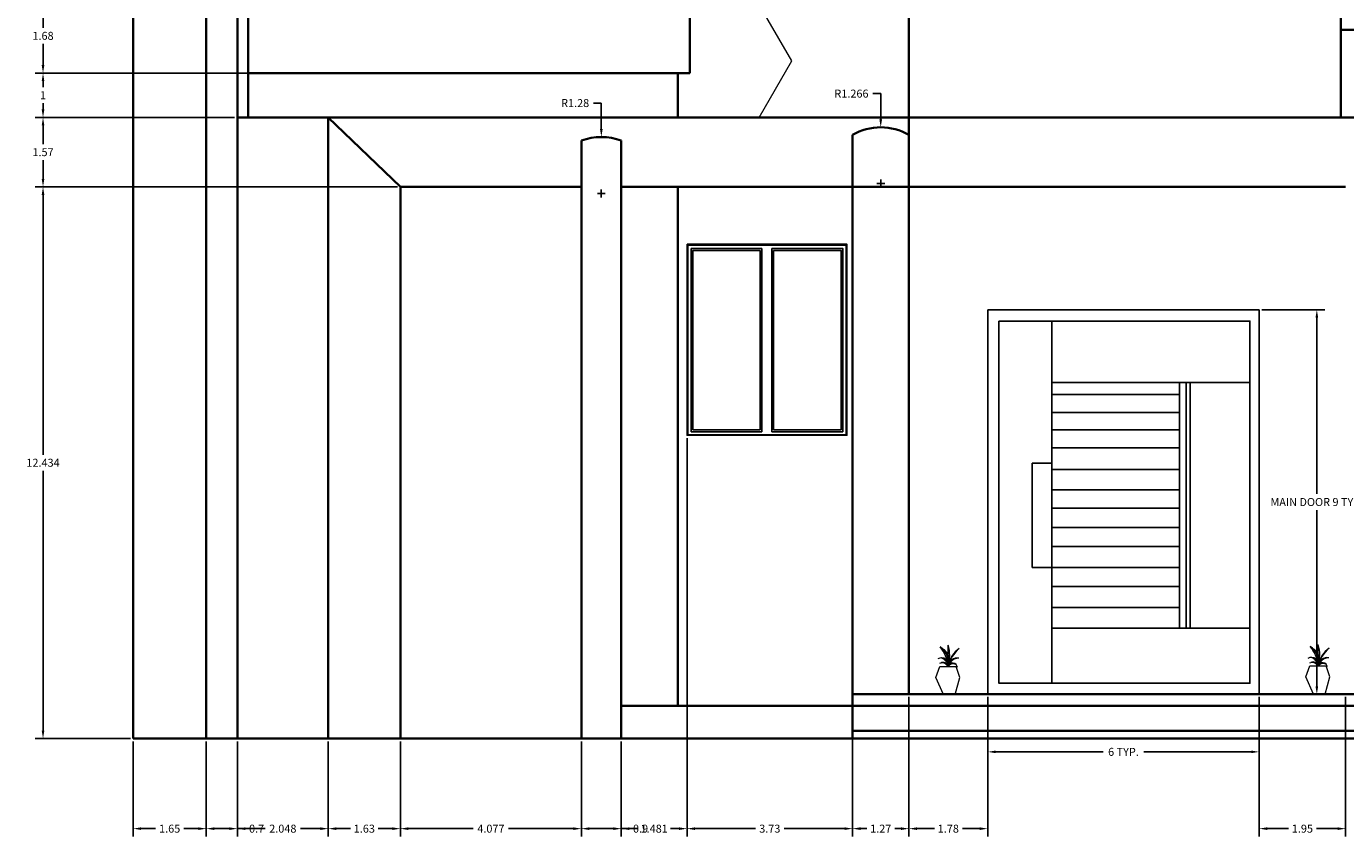
# Model space of a CAD drawing. Units: millimetres. Extents: x 2521.2 to 2565.9, y 755.2 to 798.1.
# Tile 1 of 3: x 2521.2 to 2550.9, y 755.2 to 773.4. Entities that reach past the tile are written whole.
import ezdxf

# ---------------------------------------------------------------- set-up
doc = ezdxf.new("R2010")
doc.units = ezdxf.units.MM
for name, color, linetype, lineweight in [('A-ANNO-DIMS', 2, 'Continuous', 18), ('A-DOOR', 3, 'Continuous', 25), ('A-ELEV', 7, 'Continuous', 35), ('A-GLAZ', 4, 'Continuous', 25), ('A-WALL-PATT', 8, 'Continuous', 13), ('L-PLNT', 3, 'Continuous', 18)]:
    doc.layers.add(name, color=color, linetype=linetype, lineweight=lineweight)
doc.styles.get("Standard").update_dxf_attribs({"font": 'arial.ttf'})
doc.dimstyles.get("Standard").update_dxf_attribs({"dimtxt": 0.18, "dimasz": 0.18, "dimexe": 0.18, "dimexo": 0.0625, "dimgap": 0.09, "dimtad": 0, "dimtih": 1, "dimtoh": 1, "dimdec": 4, "dimzin": 0, "dimdsep": 46, "dimtxsty": 'Standard', "dimcen": 0.09, "dimadec": 0, "dimazin": 0, "dimtfac": 1, "dimtdec": 4, "dimtofl": 0, "dimtmove": 0, "dimatfit": 3, "dimfxl": 1, "dimtolj": 1, "dimtzin": 0, "dimarcsym": 0})

# ---------------------------------------------------------------- blocks, each defined once
blk = doc.blocks.new('WIN-DOUBLE')
for p, q in [((2559.456, 776.3), (2559.456, 780.343)), ((2559.491, 780.386), (2559.491, 776.258)), ((2559.716, 776.3), (2559.716, 780.386)), ((2559.756, 776.3), (2559.756, 780.343)), ((2559.716, 776.3), (2559.716, 776.258)), ((2559.716, 776.258), (2561.319, 776.258))]:
    blk.add_line(p, q)
for points in [[(2557.805, 780.483), (2561.406, 780.483), (2561.406, 776.176), (2557.805, 776.176)], [(2557.825, 780.462), (2561.393, 780.462), (2561.393, 776.189), (2557.825, 776.189)]]:
    blk.add_lwpolyline(points, close=True)
for points in [[(2559.491, 776.258), (2557.898, 776.258), (2557.898, 780.386), (2559.491, 780.386)], [(2559.456, 776.3), (2557.936, 776.3), (2557.936, 780.343), (2559.456, 780.343)], [(2559.716, 780.386), (2561.319, 780.386), (2561.319, 776.258)], [(2559.756, 780.343), (2561.276, 780.343), (2561.276, 776.3), (2559.756, 776.3)]]:
    blk.add_lwpolyline(points)
blk = doc.blocks.new('DOOR-MAIN')
for p, q in [((2542.828, 758.373), (2542.828, 767.037)), ((2542.828, 767.037), (2548.944, 767.037)), ((2548.944, 767.037), (2548.944, 758.373)), ((2544.274, 766.783), (2544.274, 758.62)), ((2544.274, 765.396), (2548.734, 765.396)), ((2547.145, 765.132), (2544.274, 765.132)), ((2547.145, 765.396), (2547.145, 759.865)), ((2547.299, 765.396), (2547.299, 759.865)), ((2547.389, 765.396), (2547.389, 759.865)), ((2547.145, 764.725), (2544.274, 764.725)), ((2547.145, 764.331), (2544.274, 764.331)), ((2547.145, 763.924), (2544.274, 763.924)), ((2543.829, 761.227), (2543.829, 763.581)), ((2543.829, 763.581), (2544.274, 763.581)), ((2547.145, 763.441), (2544.274, 763.441)), ((2547.145, 762.983), (2544.274, 762.983)), ((2547.145, 762.564), (2544.274, 762.564)), ((2547.145, 762.131), (2544.274, 762.131)), ((2547.145, 761.699), (2544.274, 761.699)), ((2544.274, 761.227), (2543.829, 761.227)), ((2547.145, 761.227), (2544.274, 761.227)), ((2547.145, 760.804), (2544.274, 760.804)), ((2547.145, 760.33), (2544.274, 760.33)), ((2544.274, 759.865), (2548.734, 759.865))]:
    blk.add_line(p, q)
blk.add_lwpolyline([(2543.079, 766.783), (2548.734, 766.783), (2548.734, 758.62), (2543.079, 758.62)], close=True)
blk = doc.blocks.new('PLANTER')
for p, q in [((2558.646, 757.758), (2558.737, 758.005)), ((2558.737, 758.005), (2559.107, 758.005)), ((2559.189, 757.758), (2559.107, 758.005)), ((2558.817, 757.373), (2558.646, 757.758)), ((2559.08, 757.373), (2559.189, 757.758))]:
    blk.add_line(p, q)
for centre, radius, start, end in [((2558.504, 758.092), 0.427, 348.2161, 55.5831), ((2558.151, 757.944), 0.777, 5.6498, 40.0889), ((2558.161, 757.954), 0.763, 3.8104, 39.9888), ((2558.66, 758.146), 0.293, 333.1798, 63.2065), ((2558.164, 758.26), 0.796, 342.0282, 16.5628), ((2559.557, 757.89), 0.648, 126.493, 168.9551), ((2530.529, 758.527), 28.398, 358.9459, 359.9172), ((2559.736, 757.784), 0.843, 132.0051, 164.8224), ((2558.772, 758.043), 0.155, 345.7039, 120.8927), ((2558.788, 757.931), 0.154, 28.8769, 113.7957), ((2558.813, 757.985), 0.111, 10.1799, 119.9068), ((2558.697, 757.984), 0.226, 5.301, 71.0335), ((2559.127, 757.986), 0.208, 79.6534, 172.2119), ((2559.023, 757.968), 0.112, 7.4318, 155.8017), ((2559.176, 757.925), 0.266, 92.441, 162.4192), ((2559.033, 757.927), 0.136, 55.8779, 144.8755)]:
    blk.add_arc(centre, radius, start, end)
blk = doc.blocks.new('*D6')
at = {"layer": 'A-ANNO-DIMS', "color": 0, "lineweight": -2, "transparency": 16777216}
for p, q in [((2549.006, 767.037), (2550.423, 767.037)), ((2550.243, 766.857), (2550.243, 762.888)), ((2550.243, 758.553), (2550.243, 762.522)), ((2549.006, 758.373), (2550.423, 758.373))]:
    blk.add_line(p, q, dxfattribs=at)
at = {"layer": 'A-ANNO-DIMS', "color": 0, "transparency": 16777216}
for points in [[(2550.213, 766.857), (2550.273, 766.857), (2550.243, 767.037)], [(2550.213, 758.553), (2550.273, 758.553), (2550.243, 758.373)]]:
    blk.add_solid(points, dxfattribs=at)
at = {"layer": 'Defpoints', "color": 0, "transparency": 16777216}
for p in [(2548.944, 767.037), (2550.243, 767.037), (2548.944, 758.373)]:
    blk.add_point(p, dxfattribs=at)
at = {"layer": 'A-ANNO-DIMS', "color": 0, "transparency": 16777216, "insert": (2550.243, 762.705), "char_height": 0.18, "attachment_point": 5}
blk.add_mtext('\\A1;MAIN DOOR 9 TYP.', dxfattribs=at)
blk = doc.blocks.new('*D7')
at = {"layer": 'A-ANNO-DIMS', "color": 0, "lineweight": -2, "transparency": 16777216}
for p, q in [((2542.828, 758.311), (2542.828, 756.894)), ((2548.944, 758.311), (2548.944, 756.894)), ((2543.008, 757.074), (2545.427, 757.074)), ((2548.764, 757.074), (2546.344, 757.074))]:
    blk.add_line(p, q, dxfattribs=at)
at = {"layer": 'A-ANNO-DIMS', "color": 0, "transparency": 16777216}
for points in [[(2543.008, 757.104), (2543.008, 757.044), (2542.828, 757.074)], [(2548.764, 757.104), (2548.764, 757.044), (2548.944, 757.074)]]:
    blk.add_solid(points, dxfattribs=at)
at = {"layer": 'Defpoints', "color": 0, "transparency": 16777216}
for p in [(2542.828, 758.373), (2548.944, 758.373), (2548.944, 757.074)]:
    blk.add_point(p, dxfattribs=at)
at = {"layer": 'A-ANNO-DIMS', "color": 0, "transparency": 16777216, "insert": (2545.886, 757.074), "char_height": 0.18, "attachment_point": 5}
blk.add_mtext('\\A1;6 TYP.', dxfattribs=at)
blk = doc.blocks.new('*D10')
at = {"layer": 'A-ANNO-DIMS', "color": 0, "lineweight": -2, "transparency": 16777216}
for p, q in [((2529.532, 769.807), (2521.361, 769.807)), ((2521.541, 769.627), (2521.541, 763.772)), ((2521.541, 757.553), (2521.541, 763.408)), ((2523.509, 757.373), (2521.361, 757.373))]:
    blk.add_line(p, q, dxfattribs=at)
at = {"layer": 'A-ANNO-DIMS', "color": 0, "transparency": 16777216}
for points in [[(2521.511, 769.627), (2521.571, 769.627), (2521.541, 769.807)], [(2521.511, 757.553), (2521.571, 757.553), (2521.541, 757.373)]]:
    blk.add_solid(points, dxfattribs=at)
at = {"layer": 'Defpoints', "color": 0, "transparency": 16777216}
for p in [(2521.541, 769.807), (2529.594, 769.807), (2523.571, 757.373)]:
    blk.add_point(p, dxfattribs=at)
at = {"layer": 'A-ANNO-DIMS', "color": 0, "transparency": 16777216, "insert": (2521.541, 763.59), "char_height": 0.18, "attachment_point": 5}
blk.add_mtext('\\A1;12.434', dxfattribs=at)
blk = doc.blocks.new('*D11')
at = {"layer": 'A-ANNO-DIMS', "color": 0, "lineweight": -2, "transparency": 16777216}
for p, q in [((2525.857, 771.373), (2521.361, 771.373)), ((2521.541, 771.193), (2521.541, 770.772)), ((2521.541, 769.987), (2521.541, 770.408)), ((2529.532, 769.807), (2521.361, 769.807))]:
    blk.add_line(p, q, dxfattribs=at)
at = {"layer": 'A-ANNO-DIMS', "color": 0, "transparency": 16777216}
for points in [[(2521.511, 771.193), (2521.571, 771.193), (2521.541, 771.373)], [(2521.511, 769.987), (2521.571, 769.987), (2521.541, 769.807)]]:
    blk.add_solid(points, dxfattribs=at)
at = {"layer": 'Defpoints', "color": 0, "transparency": 16777216}
for p in [(2521.541, 771.373), (2525.92, 771.373), (2529.594, 769.807)]:
    blk.add_point(p, dxfattribs=at)
at = {"layer": 'A-ANNO-DIMS', "color": 0, "transparency": 16777216, "insert": (2521.541, 770.59), "char_height": 0.18, "attachment_point": 5}
blk.add_mtext('\\A1;1.57', dxfattribs=at)
blk = doc.blocks.new('*D12')
at = {"layer": 'A-ANNO-DIMS', "color": 0, "lineweight": -2, "transparency": 16777216}
for p, q in [((2536.053, 772.373), (2521.361, 772.373)), ((2521.541, 772.193), (2521.541, 772.054)), ((2521.541, 771.553), (2521.541, 771.693)), ((2525.857, 771.373), (2521.361, 771.373))]:
    blk.add_line(p, q, dxfattribs=at)
at = {"layer": 'A-ANNO-DIMS', "color": 0, "transparency": 16777216}
for points in [[(2521.511, 772.193), (2521.571, 772.193), (2521.541, 772.373)], [(2521.511, 771.553), (2521.571, 771.553), (2521.541, 771.373)]]:
    blk.add_solid(points, dxfattribs=at)
at = {"layer": 'Defpoints', "color": 0, "transparency": 16777216}
for p in [(2521.541, 772.373), (2536.116, 772.373), (2525.92, 771.373)]:
    blk.add_point(p, dxfattribs=at)
at = {"layer": 'A-ANNO-DIMS', "color": 0, "transparency": 16777216, "insert": (2521.541, 771.873), "char_height": 0.18, "attachment_point": 5}
blk.add_mtext('\\A1;1', dxfattribs=at)
blk = doc.blocks.new('*D13')
at = {"layer": 'A-ANNO-DIMS', "color": 0, "lineweight": -2, "transparency": 16777216}
for p, q in [((2536.053, 774.051), (2521.361, 774.051)), ((2521.541, 773.871), (2521.541, 773.394)), ((2521.541, 772.553), (2521.541, 773.03)), ((2536.053, 772.373), (2521.361, 772.373))]:
    blk.add_line(p, q, dxfattribs=at)
at = {"layer": 'A-ANNO-DIMS', "color": 0, "transparency": 16777216}
for points in [[(2521.511, 773.871), (2521.571, 773.871), (2521.541, 774.051)], [(2521.511, 772.553), (2521.571, 772.553), (2521.541, 772.373)]]:
    blk.add_solid(points, dxfattribs=at)
at = {"layer": 'Defpoints', "color": 0, "transparency": 16777216}
for p in [(2521.541, 774.051), (2536.116, 774.051), (2536.116, 772.373)]:
    blk.add_point(p, dxfattribs=at)
at = {"layer": 'A-ANNO-DIMS', "color": 0, "transparency": 16777216, "insert": (2521.541, 773.212), "char_height": 0.18, "attachment_point": 5}
blk.add_mtext('\\A1;1.68', dxfattribs=at)
blk = doc.blocks.new('*D35')
at = {"layer": 'A-ANNO-DIMS', "color": 0, "lineweight": -2, "transparency": 16777216}
for p, q in [((2523.571, 757.311), (2523.571, 755.163)), ((2525.22, 757.311), (2525.22, 755.163)), ((2523.751, 755.343), (2524.079, 755.343)), ((2525.04, 755.343), (2524.711, 755.343))]:
    blk.add_line(p, q, dxfattribs=at)
at = {"layer": 'A-ANNO-DIMS', "color": 0, "transparency": 16777216}
for points in [[(2523.751, 755.373), (2523.751, 755.313), (2523.571, 755.343)], [(2525.04, 755.373), (2525.04, 755.313), (2525.22, 755.343)]]:
    blk.add_solid(points, dxfattribs=at)
at = {"layer": 'Defpoints', "color": 0, "transparency": 16777216}
for p in [(2523.571, 757.373), (2525.22, 757.373), (2525.22, 755.343)]:
    blk.add_point(p, dxfattribs=at)
at = {"layer": 'A-ANNO-DIMS', "color": 0, "transparency": 16777216, "insert": (2524.395, 755.343), "char_height": 0.18, "attachment_point": 5}
blk.add_mtext('\\A1;1.65', dxfattribs=at)
blk = doc.blocks.new('*D36')
at = {"layer": 'A-ANNO-DIMS', "color": 0, "lineweight": -2, "transparency": 16777216}
for p, q in [((2525.22, 757.311), (2525.22, 755.163)), ((2525.92, 757.311), (2525.92, 755.163)), ((2525.4, 755.343), (2525.74, 755.343)), ((2525.92, 755.343), (2526.1, 755.343))]:
    blk.add_line(p, q, dxfattribs=at)
at = {"layer": 'A-ANNO-DIMS', "color": 0, "transparency": 16777216}
for points in [[(2525.4, 755.373), (2525.4, 755.313), (2525.22, 755.343)], [(2525.74, 755.373), (2525.74, 755.313), (2525.92, 755.343)]]:
    blk.add_solid(points, dxfattribs=at)
at = {"layer": 'Defpoints', "color": 0, "transparency": 16777216}
for p in [(2525.22, 757.373), (2525.92, 757.373), (2525.92, 755.343)]:
    blk.add_point(p, dxfattribs=at)
at = {"layer": 'A-ANNO-DIMS', "color": 0, "transparency": 16777216, "insert": (2526.354, 755.343), "char_height": 0.18, "attachment_point": 5}
blk.add_mtext('\\A1;0.7', dxfattribs=at)
blk = doc.blocks.new('*D37')
at = {"layer": 'A-ANNO-DIMS', "color": 0, "lineweight": -2, "transparency": 16777216}
for p, q in [((2525.92, 757.311), (2525.92, 755.163)), ((2527.968, 757.311), (2527.968, 755.163)), ((2526.1, 755.343), (2526.548, 755.343)), ((2527.788, 755.343), (2527.339, 755.343))]:
    blk.add_line(p, q, dxfattribs=at)
at = {"layer": 'A-ANNO-DIMS', "color": 0, "transparency": 16777216}
for points in [[(2526.1, 755.373), (2526.1, 755.313), (2525.92, 755.343)], [(2527.788, 755.373), (2527.788, 755.313), (2527.968, 755.343)]]:
    blk.add_solid(points, dxfattribs=at)
at = {"layer": 'Defpoints', "color": 0, "transparency": 16777216}
for p in [(2525.92, 757.373), (2527.968, 757.373), (2527.968, 755.343)]:
    blk.add_point(p, dxfattribs=at)
at = {"layer": 'A-ANNO-DIMS', "color": 0, "transparency": 16777216, "insert": (2526.944, 755.343), "char_height": 0.18, "attachment_point": 5}
blk.add_mtext('\\A1;2.048', dxfattribs=at)
blk = doc.blocks.new('*D38')
at = {"layer": 'A-ANNO-DIMS', "color": 0, "lineweight": -2, "transparency": 16777216}
for p, q in [((2527.968, 757.311), (2527.968, 755.163)), ((2529.594, 757.311), (2529.594, 755.163)), ((2528.148, 755.343), (2528.466, 755.343)), ((2529.414, 755.343), (2529.096, 755.343))]:
    blk.add_line(p, q, dxfattribs=at)
at = {"layer": 'A-ANNO-DIMS', "color": 0, "transparency": 16777216}
for points in [[(2528.148, 755.373), (2528.148, 755.313), (2527.968, 755.343)], [(2529.414, 755.373), (2529.414, 755.313), (2529.594, 755.343)]]:
    blk.add_solid(points, dxfattribs=at)
at = {"layer": 'Defpoints', "color": 0, "transparency": 16777216}
for p in [(2527.968, 757.373), (2529.594, 757.373), (2529.594, 755.343)]:
    blk.add_point(p, dxfattribs=at)
at = {"layer": 'A-ANNO-DIMS', "color": 0, "transparency": 16777216, "insert": (2528.781, 755.343), "char_height": 0.18, "attachment_point": 5}
blk.add_mtext('\\A1;1.63', dxfattribs=at)
blk = doc.blocks.new('*D39')
at = {"layer": 'A-ANNO-DIMS', "color": 0, "lineweight": -2, "transparency": 16777216}
for p, q in [((2529.594, 757.311), (2529.594, 755.163)), ((2533.671, 757.311), (2533.671, 755.163)), ((2529.774, 755.343), (2531.235, 755.343)), ((2533.491, 755.343), (2532.03, 755.343))]:
    blk.add_line(p, q, dxfattribs=at)
at = {"layer": 'A-ANNO-DIMS', "color": 0, "transparency": 16777216}
for points in [[(2529.774, 755.373), (2529.774, 755.313), (2529.594, 755.343)], [(2533.491, 755.373), (2533.491, 755.313), (2533.671, 755.343)]]:
    blk.add_solid(points, dxfattribs=at)
at = {"layer": 'Defpoints', "color": 0, "transparency": 16777216}
for p in [(2529.594, 757.373), (2533.671, 757.373), (2533.671, 755.343)]:
    blk.add_point(p, dxfattribs=at)
at = {"layer": 'A-ANNO-DIMS', "color": 0, "transparency": 16777216, "insert": (2531.633, 755.343), "char_height": 0.18, "attachment_point": 5}
blk.add_mtext('\\A1;4.077', dxfattribs=at)
blk = doc.blocks.new('*D40')
at = {"layer": 'A-ANNO-DIMS', "color": 0, "lineweight": -2, "transparency": 16777216}
for p, q in [((2533.671, 757.311), (2533.671, 755.163)), ((2534.571, 757.311), (2534.571, 755.163)), ((2533.851, 755.343), (2534.391, 755.343)), ((2534.571, 755.343), (2534.751, 755.343))]:
    blk.add_line(p, q, dxfattribs=at)
at = {"layer": 'A-ANNO-DIMS', "color": 0, "transparency": 16777216}
for points in [[(2533.851, 755.373), (2533.851, 755.313), (2533.671, 755.343)], [(2534.391, 755.373), (2534.391, 755.313), (2534.571, 755.343)]]:
    blk.add_solid(points, dxfattribs=at)
at = {"layer": 'Defpoints', "color": 0, "transparency": 16777216}
for p in [(2533.671, 757.373), (2534.571, 757.373), (2534.571, 755.343)]:
    blk.add_point(p, dxfattribs=at)
at = {"layer": 'A-ANNO-DIMS', "color": 0, "transparency": 16777216, "insert": (2535.005, 755.343), "char_height": 0.18, "attachment_point": 5}
blk.add_mtext('\\A1;0.9', dxfattribs=at)
blk = doc.blocks.new('*D41')
at = {"layer": 'A-ANNO-DIMS', "color": 0, "lineweight": -2, "transparency": 16777216}
for p, q in [((2536.052, 764.146), (2536.052, 755.163)), ((2534.571, 757.311), (2534.571, 755.163)), ((2534.751, 755.343), (2534.944, 755.343)), ((2535.872, 755.343), (2535.679, 755.343))]:
    blk.add_line(p, q, dxfattribs=at)
at = {"layer": 'A-ANNO-DIMS', "color": 0, "transparency": 16777216}
for points in [[(2534.751, 755.373), (2534.751, 755.313), (2534.571, 755.343)], [(2535.872, 755.373), (2535.872, 755.313), (2536.052, 755.343)]]:
    blk.add_solid(points, dxfattribs=at)
at = {"layer": 'Defpoints', "color": 0, "transparency": 16777216}
for p in [(2536.052, 764.209), (2534.571, 757.373), (2536.052, 755.343)]:
    blk.add_point(p, dxfattribs=at)
at = {"layer": 'A-ANNO-DIMS', "color": 0, "transparency": 16777216, "insert": (2535.312, 755.343), "char_height": 0.18, "attachment_point": 5}
blk.add_mtext('\\A1;1.481', dxfattribs=at)
blk = doc.blocks.new('*D42')
at = {"layer": 'A-ANNO-DIMS', "color": 0, "lineweight": -2, "transparency": 16777216}
for p, q in [((2536.052, 764.146), (2536.052, 755.163)), ((2539.782, 758.311), (2539.782, 755.163)), ((2536.232, 755.343), (2537.594, 755.343)), ((2539.602, 755.343), (2538.241, 755.343))]:
    blk.add_line(p, q, dxfattribs=at)
at = {"layer": 'A-ANNO-DIMS', "color": 0, "transparency": 16777216}
for points in [[(2536.232, 755.373), (2536.232, 755.313), (2536.052, 755.343)], [(2539.602, 755.373), (2539.602, 755.313), (2539.782, 755.343)]]:
    blk.add_solid(points, dxfattribs=at)
at = {"layer": 'Defpoints', "color": 0, "transparency": 16777216}
for p in [(2536.052, 764.209), (2539.782, 758.373), (2539.782, 755.343)]:
    blk.add_point(p, dxfattribs=at)
at = {"layer": 'A-ANNO-DIMS', "color": 0, "transparency": 16777216, "insert": (2537.917, 755.343), "char_height": 0.18, "attachment_point": 5}
blk.add_mtext('\\A1;3.73', dxfattribs=at)
blk = doc.blocks.new('*D43')
at = {"layer": 'A-ANNO-DIMS', "color": 0, "lineweight": -2, "transparency": 16777216}
for p, q in [((2539.782, 758.311), (2539.782, 755.163)), ((2541.052, 758.311), (2541.052, 755.163)), ((2539.962, 755.343), (2540.102, 755.343)), ((2540.872, 755.343), (2540.733, 755.343))]:
    blk.add_line(p, q, dxfattribs=at)
at = {"layer": 'A-ANNO-DIMS', "color": 0, "transparency": 16777216}
for points in [[(2539.962, 755.373), (2539.962, 755.313), (2539.782, 755.343)], [(2540.872, 755.373), (2540.872, 755.313), (2541.052, 755.343)]]:
    blk.add_solid(points, dxfattribs=at)
at = {"layer": 'Defpoints', "color": 0, "transparency": 16777216}
for p in [(2539.782, 758.373), (2541.052, 758.373), (2541.052, 755.343)]:
    blk.add_point(p, dxfattribs=at)
at = {"layer": 'A-ANNO-DIMS', "color": 0, "transparency": 16777216, "insert": (2540.417, 755.343), "char_height": 0.18, "attachment_point": 5}
blk.add_mtext('\\A1;1.27', dxfattribs=at)
blk = doc.blocks.new('*D44')
at = {"layer": 'A-ANNO-DIMS', "color": 0, "lineweight": -2, "transparency": 16777216}
for p, q in [((2541.052, 758.311), (2541.052, 755.163)), ((2542.828, 758.311), (2542.828, 755.163)), ((2541.232, 755.343), (2541.625, 755.343)), ((2542.648, 755.343), (2542.256, 755.343))]:
    blk.add_line(p, q, dxfattribs=at)
at = {"layer": 'A-ANNO-DIMS', "color": 0, "transparency": 16777216}
for points in [[(2541.232, 755.373), (2541.232, 755.313), (2541.052, 755.343)], [(2542.648, 755.373), (2542.648, 755.313), (2542.828, 755.343)]]:
    blk.add_solid(points, dxfattribs=at)
at = {"layer": 'Defpoints', "color": 0, "transparency": 16777216}
for p in [(2541.052, 758.373), (2542.828, 758.373), (2542.828, 755.343)]:
    blk.add_point(p, dxfattribs=at)
at = {"layer": 'A-ANNO-DIMS', "color": 0, "transparency": 16777216, "insert": (2541.94, 755.343), "char_height": 0.18, "attachment_point": 5}
blk.add_mtext('\\A1;1.78', dxfattribs=at)
blk = doc.blocks.new('*D45')
at = {"layer": 'A-ANNO-DIMS', "color": 0, "lineweight": -2, "transparency": 16777216}
for p, q in [((2548.944, 758.311), (2548.944, 755.163)), ((2550.892, 758.311), (2550.892, 755.163)), ((2549.124, 755.343), (2549.602, 755.343)), ((2550.712, 755.343), (2550.234, 755.343))]:
    blk.add_line(p, q, dxfattribs=at)
at = {"layer": 'A-ANNO-DIMS', "color": 0, "transparency": 16777216}
for points in [[(2549.124, 755.373), (2549.124, 755.313), (2548.944, 755.343)], [(2550.712, 755.373), (2550.712, 755.313), (2550.892, 755.343)]]:
    blk.add_solid(points, dxfattribs=at)
at = {"layer": 'Defpoints', "color": 0, "transparency": 16777216}
for p in [(2548.944, 758.373), (2550.892, 758.373), (2550.892, 755.343)]:
    blk.add_point(p, dxfattribs=at)
at = {"layer": 'A-ANNO-DIMS', "color": 0, "transparency": 16777216, "insert": (2549.918, 755.343), "char_height": 0.18, "attachment_point": 5}
blk.add_mtext('\\A1;1.95', dxfattribs=at)
blk = doc.blocks.new('*D46')
at = {"layer": 'A-ANNO-DIMS', "color": 0, "lineweight": -2, "transparency": 16777216}
for p, q in [((2550.891519, 758.310917), (2550.891519, 755.163417)), ((2552.163561, 758.310917), (2552.163561, 755.163417)), ((2550.711519, 755.343417), (2550.531519, 755.343417)), ((2552.343561, 755.343417), (2552.523561, 755.343417))]:
    blk.add_line(p, q, dxfattribs=at)
at = {"layer": 'A-ANNO-DIMS', "color": 0, "transparency": 16777216}
for points in [[(2550.711519, 755.373417), (2550.711519, 755.313417), (2550.891519, 755.343417)], [(2552.343561, 755.373417), (2552.343561, 755.313417), (2552.163561, 755.343417)]]:
    blk.add_solid(points, dxfattribs=at)
at = {"layer": 'Defpoints', "color": 0, "transparency": 16777216}
for p in [(2550.891519, 758.373417), (2552.163561, 758.373417), (2552.163561, 755.343417)]:
    blk.add_point(p, dxfattribs=at)
at = {"layer": 'A-ANNO-DIMS', "color": 0, "transparency": 16777216, "insert": (2551.52754, 755.343417), "char_height": 0.18, "attachment_point": 5}
blk.add_mtext('\\A1;1.272', dxfattribs=at)
blk = doc.blocks.new('*D68')
at = {"layer": 'A-ANNO-DIMS', "color": 0, "lineweight": -2, "transparency": 16777216}
for p, q in [((2533.941, 771.697), (2534.121, 771.697)), ((2534.121, 771.697), (2534.121, 771.111)), ((2534.031, 769.656), (2534.211, 769.656)), ((2534.121, 769.566), (2534.121, 769.746))]:
    blk.add_line(p, q, dxfattribs=at)
at = {"layer": 'A-ANNO-DIMS', "color": 0, "transparency": 16777216}
blk.add_solid([(2534.151, 771.111), (2534.091, 771.111), (2534.121, 770.931)], dxfattribs=at)
at = {"layer": 'Defpoints', "color": 0, "transparency": 16777216}
for p in [(2534.121, 770.931), (2534.121, 769.656)]:
    blk.add_point(p, dxfattribs=at)
at = {"layer": 'A-ANNO-DIMS', "color": 0, "transparency": 16777216, "insert": (2533.531, 771.697), "char_height": 0.18, "attachment_point": 5}
blk.add_mtext('\\A1;R1.28', dxfattribs=at)
blk = doc.blocks.new('*D69')
at = {"layer": 'A-ANNO-DIMS', "color": 0, "lineweight": -2, "transparency": 16777216}
for p, q in [((2540.237, 771.91), (2540.417, 771.91)), ((2540.417, 771.91), (2540.417, 771.33)), ((2540.417, 769.794), (2540.417, 769.974)), ((2540.327, 769.884), (2540.507, 769.884))]:
    blk.add_line(p, q, dxfattribs=at)
at = {"layer": 'A-ANNO-DIMS', "color": 0, "transparency": 16777216}
blk.add_solid([(2540.447, 771.33), (2540.387, 771.33), (2540.417, 771.15)], dxfattribs=at)
at = {"layer": 'Defpoints', "color": 0, "transparency": 16777216}
for p in [(2540.417, 771.15), (2540.417, 769.884)]:
    blk.add_point(p, dxfattribs=at)
at = {"layer": 'A-ANNO-DIMS', "color": 0, "transparency": 16777216, "insert": (2539.757, 771.91), "char_height": 0.18, "attachment_point": 5}
blk.add_mtext('\\A1;R1.266', dxfattribs=at)

msp = doc.modelspace()

# ---------------------------------------------------------------- hatches: boundary and pattern name
at = {"layer": 'A-WALL-PATT'}
h = msp.add_hatch(dxfattribs=at)
h.set_pattern_fill('HEX', color=256)
h.paths.add_polyline_path([(2543.5368, 792.7443), (2533.5167, 792.7443), (2533.5167, 789.7118), (2533.5167, 787.2308), (2543.5368, 787.2308)])
h.paths.add_polyline_path([(2541.0523, 787.2308), (2534.0845, 787.2308), (2534.0845, 782.5843), (2534.0845, 780.4594), (2534.0845, 775.7444), (2536.0482, 775.7444), (2536.0482, 775.5347), (2535.8852, 775.5347), (2535.8852, 774.0509), (2536.1156, 774.0509), (2536.1156, 772.3734), (2535.8428, 772.3734), (2535.8428, 771.3734), (2541.0523, 771.3734), (2541.0523, 782.5843)])

# ---------------------------------------------------------------- linework, layer by layer
at = {"layer": 'A-ELEV'}
for p, q in [((2523.5711, 757.3734), (2523.5711, 795.8762)), ((2525.2197, 787.3734), (2525.2197, 757.3734)), ((2525.9197, 757.3734), (2525.9197, 787.2308)), ((2541.0523, 770.9792), (2541.0523, 782.5843)), ((2526.1636, 772.3734), (2526.1636, 774.7183)), ((2536.1156, 772.3734), (2536.1156, 774.0509)), ((2550.7859, 771.3734), (2550.7859, 773.6725)), ((2550.7859, 773.3478), (2555.0021, 773.3478)), ((2526.1636, 771.3734), (2526.1636, 772.3734)), ((2526.1636, 772.3734), (2535.8428, 772.3734)), ((2535.8428, 772.3734), (2535.8428, 771.3734)), ((2535.8428, 772.3734), (2536.1156, 772.3734)), ((2525.9827, 771.3734), (2525.9197, 771.3734)), ((2534.5711, 771.3734), (2525.9827, 771.3734)), ((2527.9678, 771.3734), (2527.9678, 757.3734)), ((2527.9678, 771.3734), (2529.5941, 769.807)), ((2534.5711, 771.3734), (2550.7859, 771.3734)), ((2550.7859, 771.3734), (2556.5711, 771.3734)), ((2533.671, 770.8494), (2533.671, 757.3734)), ((2534.5711, 770.8494), (2534.5711, 757.3734)), ((2539.7823, 758.3734), (2539.7823, 770.9792)), ((2541.0523, 770.9792), (2541.0523, 758.3734)), ((2529.5941, 769.807), (2533.671, 769.807)), ((2529.5941, 769.807), (2529.5941, 757.3734)), ((2535.8411, 769.807), (2534.5711, 769.807)), ((2535.8411, 769.807), (2550.8915, 769.807)), ((2535.8411, 769.807), (2535.8411, 758.1133)), ((2539.7823, 758.3734), (2539.7823, 757.3734)), ((2539.7823, 758.3734), (2556.5711, 758.3734)), ((2539.7823, 758.1133), (2534.5711, 758.1133)), ((2539.7823, 758.1133), (2556.5711, 758.1133)), ((2539.7823, 757.5506), (2556.5711, 757.5506)), ((2523.5711, 757.3734), (2563.5711, 757.3734))]:
    msp.add_line(p, q, dxfattribs=at)
for centre, radius, start, end in [((2540.4173, 769.8841), 1.2659, 59.8929, 120.1071), ((2534.121, 769.6562), 1.2753, 69.33582, 110.66418)]:
    msp.add_arc(centre, radius, start, end, dxfattribs=at)

# ---------------------------------------------------------------- block references
at = {"layer": 'A-DOOR'}
msp.add_blockref('DOOR-MAIN', (0, 0), dxfattribs=at)
at = {"layer": 'A-GLAZ'}
msp.add_blockref('WIN-DOUBLE', (-21.7526, -11.9678), dxfattribs=at)
at = {"layer": 'L-PLNT'}
for p in [(-8.6515, 1.0042), (-16.9888, 0.9949)]:
    msp.add_blockref('PLANTER', p, dxfattribs=at)

# ---------------------------------------------------------------- dimensions: what is measured, and where the dimension line sits
at = {"layer": 'A-ANNO-DIMS'}
for base, p1, p2, override, picture, middle in [((2521.5411, 774.0509), (2536.1156, 772.3734), (2536.1156, 774.0509), {"dimdec": 2, "dimlfac": 1, "dimrnd": 0, "dimzin": 0, "dimdsep": 46, "dimlunit": 2}, '*D13', (2521.5411, 773.2122)), ((2521.5411, 772.3734), (2525.9197, 771.3734), (2536.1156, 772.3734), {"dimdec": 0, "dimlfac": 1, "dimrnd": 0, "dimzin": 0, "dimdsep": 46, "dimlunit": 2}, '*D12', (2521.5411, 771.8734)), ((2521.5411, 771.3734), (2529.5941, 769.807), (2525.9197, 771.3734), {"dimdec": 2, "dimlfac": 1, "dimrnd": 0, "dimzin": 0, "dimdsep": 46, "dimlunit": 2}, '*D11', (2521.5411, 770.5902)), ((2521.5411, 769.807), (2523.5711, 757.3734), (2529.5941, 769.807), {"dimdec": 3, "dimlfac": 1, "dimrnd": 0, "dimzin": 0, "dimdsep": 46, "dimlunit": 2}, '*D10', (2521.5411, 763.5902))]:
    dim = msp.add_linear_dim(base=base, p1=p1, p2=p2, angle=90, dimstyle='Standard', override=override, dxfattribs=at)
    dim.commit()
    dim.dimension.update_dxf_attribs({"geometry": picture, "text_midpoint": middle})
for center, mpoint, override, picture, middle in [((2540.4173, 769.8841), (2540.417, 771.15), {"dimdec": 3, "dimlfac": 1, "dimrnd": 0, "dimzin": 0, "dimdsep": 46, "dimlunit": 2}, '*D69', (2539.7571, 771.9095)), ((2534.121, 769.6562), (2534.121, 770.9314), {"dimdec": 2, "dimlfac": 1, "dimrnd": 0, "dimzin": 0, "dimdsep": 46, "dimlunit": 2}, '*D68', (2533.5309, 771.6966))]:
    dim = msp.add_radius_dim(center=center, mpoint=mpoint, dimstyle='Standard', override=override, dxfattribs=at)
    dim.commit()
    dim.dimension.update_dxf_attribs({"geometry": picture, "text_midpoint": middle, "dimtype": 164})
dim = msp.add_linear_dim(base=(2550.2434, 767.0367), p1=(2548.9439, 758.3734), p2=(2548.9439, 767.0367), angle=90, text='MAIN DOOR <> TYP.', dimstyle='Standard', override={"dimdec": 0, "dimlfac": 1, "dimrnd": 0, "dimzin": 0, "dimdsep": 46, "dimlunit": 2}, dxfattribs=at)
dim.commit()
dim.dimension.update_dxf_attribs({"geometry": '*D6', "text_midpoint": (2550.2434, 762.7051)})
for base, p1, p2, override, picture, middle in [((2536.0522, 755.3434), (2534.5711, 757.3734), (2536.0522, 764.2086), {"dimdec": 3, "dimlfac": 1, "dimrnd": 0, "dimzin": 0, "dimdsep": 46, "dimlunit": 2}, '*D41', (2535.3116, 755.3434)), ((2539.7823, 755.3434), (2536.0522, 764.2086), (2539.7823, 758.3734), {"dimdec": 2, "dimlfac": 1, "dimrnd": 0, "dimzin": 0, "dimdsep": 46, "dimlunit": 2}, '*D42', (2537.9172, 755.3434)), ((2541.0523, 755.3434), (2539.7823, 758.3734), (2541.0523, 758.3734), {"dimdec": 2, "dimlfac": 1, "dimrnd": 0, "dimzin": 0, "dimdsep": 46, "dimlunit": 2}, '*D43', (2540.4173, 755.3434)), ((2542.8278, 755.3434), (2541.0523, 758.3734), (2542.8278, 758.3734), {"dimdec": 2, "dimlfac": 1, "dimrnd": 0, "dimzin": 0, "dimdsep": 46, "dimlunit": 2}, '*D44', (2541.94, 755.3434)), ((2550.8915, 755.3434), (2548.9439, 758.3734), (2550.8915, 758.3734), {"dimdec": 2, "dimlfac": 1, "dimrnd": 0, "dimzin": 0, "dimdsep": 46, "dimlunit": 2}, '*D45', (2549.9177, 755.3434)), ((2552.1636, 755.3434), (2550.8915, 758.3734), (2552.1636, 758.3734), {"dimdec": 3, "dimlfac": 1, "dimrnd": 0, "dimzin": 0, "dimdsep": 46, "dimlunit": 2}, '*D46', (2551.5275, 755.3434)), ((2525.2197, 755.3434), (2523.5711, 757.3734), (2525.2197, 757.3734), {"dimdec": 2, "dimlfac": 1, "dimrnd": 0, "dimzin": 0, "dimdsep": 46, "dimlunit": 2}, '*D35', (2524.3954, 755.3434)), ((2525.9197, 755.3434), (2525.2197, 757.3734), (2525.9197, 757.3734), {"dimdec": 1, "dimlfac": 1, "dimrnd": 0, "dimzin": 0, "dimdsep": 46, "dimlunit": 2}, '*D36', (2526.3535, 755.3434)), ((2527.9678, 755.3434), (2525.9197, 757.3734), (2527.9678, 757.3734), {"dimdec": 3, "dimlfac": 1, "dimrnd": 0, "dimzin": 0, "dimdsep": 46, "dimlunit": 2}, '*D37', (2526.9437, 755.3434)), ((2529.5941, 755.3434), (2527.9678, 757.3734), (2529.5941, 757.3734), {"dimdec": 2, "dimlfac": 1, "dimrnd": 0, "dimzin": 0, "dimdsep": 46, "dimlunit": 2}, '*D38', (2528.7809, 755.3434)), ((2533.671, 755.3434), (2529.5941, 757.3734), (2533.671, 757.3734), {"dimdec": 3, "dimlfac": 1, "dimrnd": 0, "dimzin": 0, "dimdsep": 46, "dimlunit": 2}, '*D39', (2531.6326, 755.3434)), ((2534.5711, 755.3434), (2533.671, 757.3734), (2534.5711, 757.3734), {"dimdec": 1, "dimlfac": 1, "dimrnd": 0, "dimzin": 0, "dimdsep": 46, "dimlunit": 2}, '*D40', (2535.0051, 755.3434))]:
    dim = msp.add_linear_dim(base=base, p1=p1, p2=p2, dimstyle='Standard', override=override, dxfattribs=at)
    dim.commit()
    dim.dimension.update_dxf_attribs({"geometry": picture, "text_midpoint": middle})
dim = msp.add_linear_dim(base=(2548.9439, 757.0739), p1=(2542.8278, 758.3734), p2=(2548.9439, 758.3734), text='<> TYP.', dimstyle='Standard', override={"dimdec": 0, "dimlfac": 1, "dimrnd": 0, "dimzin": 0, "dimdsep": 46, "dimlunit": 2}, dxfattribs=at)
dim.commit()
dim.dimension.update_dxf_attribs({"geometry": '*D7', "text_midpoint": (2545.8858, 757.0739)})

doc.saveas('drawing.dxf')
